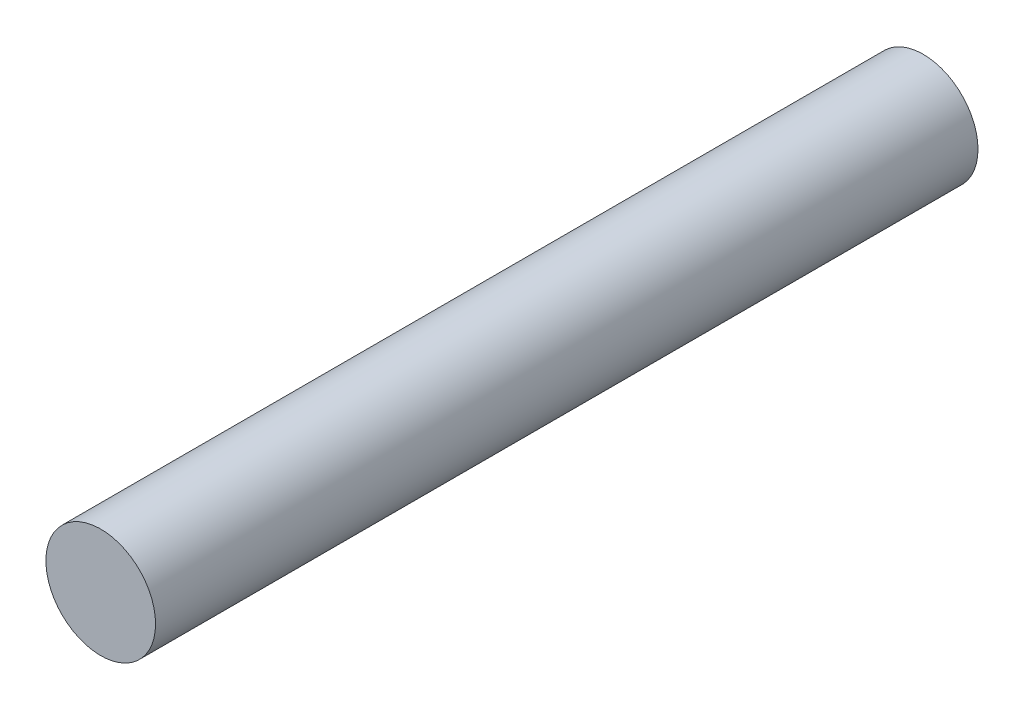
ISO-10303-21;
HEADER;
FILE_DESCRIPTION(('STEP AP214'),'2;1');
FILE_NAME('part.step','',(''),(''),'','','');
FILE_SCHEMA(('AUTOMOTIVE_DESIGN { 1 0 10303 214 1 1 1 1 }'));
ENDSEC;
DATA;
#1=APPLICATION_CONTEXT('core data for automotive mechanical design processes');
#2=APPLICATION_PROTOCOL_DEFINITION('international standard','automotive_design',2000,#1);
#3=PRODUCT_CONTEXT('',#1,'mechanical');
#4=PRODUCT('Part','Part','',(#3));
#5=PRODUCT_RELATED_PRODUCT_CATEGORY('part','',(#4));
#6=PRODUCT_DEFINITION_FORMATION('','',#4);
#7=PRODUCT_DEFINITION_CONTEXT('part definition',#1,'design');
#8=PRODUCT_DEFINITION('design','',#6,#7);
#9=PRODUCT_DEFINITION_SHAPE('','',#8);
#10=(LENGTH_UNIT() NAMED_UNIT(*) SI_UNIT(.MILLI.,.METRE.));
#11=(NAMED_UNIT(*) PLANE_ANGLE_UNIT() SI_UNIT($,.RADIAN.));
#12=(NAMED_UNIT(*) SI_UNIT($,.STERADIAN.) SOLID_ANGLE_UNIT());
#13=UNCERTAINTY_MEASURE_WITH_UNIT(LENGTH_MEASURE(1.E-05),#10,'distance_accuracy_value','');
#14=(GEOMETRIC_REPRESENTATION_CONTEXT(3) GLOBAL_UNCERTAINTY_ASSIGNED_CONTEXT((#13)) GLOBAL_UNIT_ASSIGNED_CONTEXT((#10,
#11,#12)) REPRESENTATION_CONTEXT('',''));
#15=CARTESIAN_POINT('',(0.,0.,0.));
#16=DIRECTION('',(0.,0.,1.));
#17=DIRECTION('',(1.,0.,0.));
#18=AXIS2_PLACEMENT_3D('',#15,#16,#17);
#19=CARTESIAN_POINT('',(0.,0.,30.));
#20=DIRECTION('',(0.,0.,-1.));
#21=DIRECTION('',(-1.,0.,0.));
#22=AXIS2_PLACEMENT_3D('',#19,#20,#21);
#23=CYLINDRICAL_SURFACE('',#22,2.);
#24=CARTESIAN_POINT('',(0.,0.,30.));
#25=DIRECTION('',(0.,0.,1.));
#26=DIRECTION('',(1.,0.,0.));
#27=AXIS2_PLACEMENT_3D('',#24,#25,#26);
#28=CIRCLE('',#27,2.);
#29=CARTESIAN_POINT('',(2.,0.,30.));
#30=VERTEX_POINT('',#29);
#31=EDGE_CURVE('E10',#30,#30,#28,.T.);
#32=ORIENTED_EDGE('',*,*,#31,.F.);
#33=EDGE_LOOP('',(#32));
#34=FACE_BOUND('',#33,.T.);
#35=CARTESIAN_POINT('',(0.,0.,0.));
#36=DIRECTION('',(0.,0.,1.));
#37=DIRECTION('',(1.,0.,0.));
#38=AXIS2_PLACEMENT_3D('',#35,#36,#37);
#39=CIRCLE('',#38,2.);
#40=CARTESIAN_POINT('',(2.,0.,0.));
#41=VERTEX_POINT('',#40);
#42=EDGE_CURVE('E37',#41,#41,#39,.T.);
#43=ORIENTED_EDGE('',*,*,#42,.T.);
#44=EDGE_LOOP('',(#43));
#45=FACE_BOUND('',#44,.T.);
#46=ADVANCED_FACE('F40',(#34,#45),#23,.T.);
#47=CARTESIAN_POINT('',(0.,0.,30.));
#48=DIRECTION('',(0.,0.,1.));
#49=DIRECTION('',(1.,0.,0.));
#50=AXIS2_PLACEMENT_3D('',#47,#48,#49);
#51=PLANE('',#50);
#52=ORIENTED_EDGE('',*,*,#31,.T.);
#53=EDGE_LOOP('',(#52));
#54=FACE_BOUND('',#53,.T.);
#55=ADVANCED_FACE('F55',(#54),#51,.T.);
#56=CARTESIAN_POINT('',(0.,0.,0.));
#57=DIRECTION('',(0.,0.,1.));
#58=DIRECTION('',(1.,0.,0.));
#59=AXIS2_PLACEMENT_3D('',#56,#57,#58);
#60=PLANE('',#59);
#61=ORIENTED_EDGE('',*,*,#42,.F.);
#62=EDGE_LOOP('',(#61));
#63=FACE_BOUND('',#62,.T.);
#64=ADVANCED_FACE('F49',(#63),#60,.F.);
#65=CLOSED_SHELL('',(#46,#55,#64));
#66=MANIFOLD_SOLID_BREP('B2',#65);
#67=ADVANCED_BREP_SHAPE_REPRESENTATION('',(#18,#66),#14);
#68=SHAPE_DEFINITION_REPRESENTATION(#9,#67);
ENDSEC;
END-ISO-10303-21;
